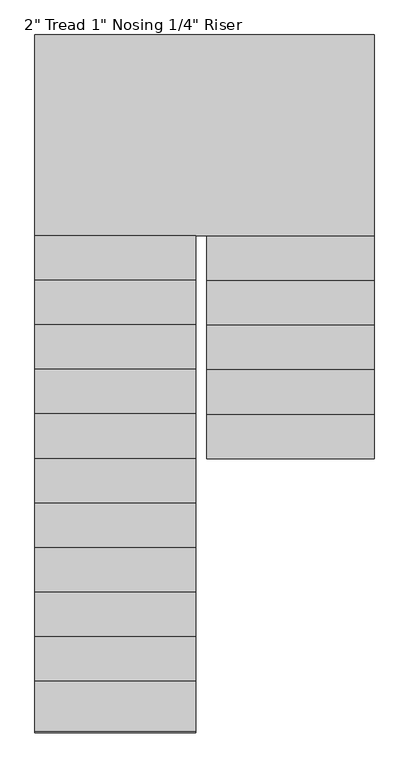
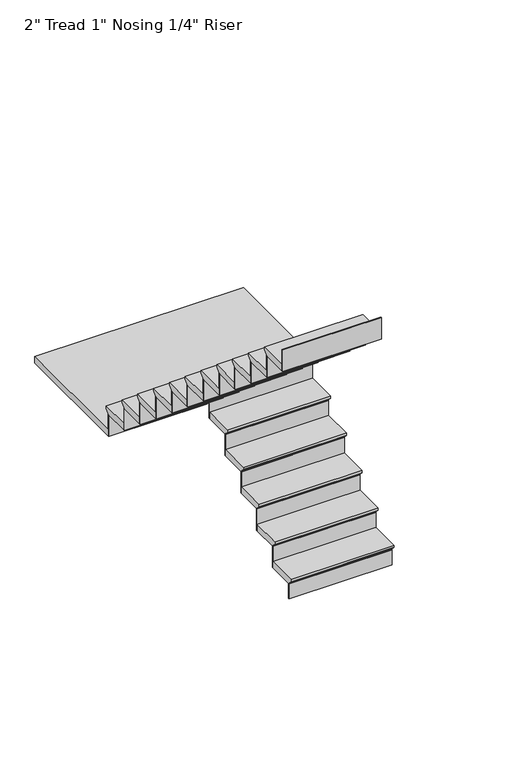
"""IFC4 building model written with IfcOpenShell, lengths in millimetres: stair flight geometry."""

from ifc_helpers import new_model, si_unit, origin, place, context, project, spatial, faceted_brep, source, transform, mapped, element, save


def stair_flight_2b9b7e9b(model_context):
    return source(origin(), model_context, "Body", "Brep", [
        faceted_brep([(-3749.597125, 2714.6319226, 150.2833333), (-3749.597125, 2714.6319226, 169.3333333), (-4512.2136682, 2714.6319226, 169.3333333), (-4512.2136682, 2714.6319226, 150.2833333), (-3749.597125, 2740.0319226, 124.8833333), (-4512.2136682, 2740.0319226, 124.8833333), (-3749.597125, 2943.2319226, 169.3333333), (-4512.2136682, 2943.2319226, 169.3333333), (-4512.2136682, 2740.0319226, 118.5333333), (-4512.2136682, 2943.2319226, 118.5333333), (-3749.597125, 2943.2319226, 118.5333333), (-3749.597125, 2740.0319226, 118.5333333)], [[[0, 1, 2, 3]], [[4, 0, 3, 5]], [[2, 1, 6, 7]], [[8, 9, 10, 11]], [[2, 7, 9, 8, 5, 3]], [[8, 11, 4, 5]], [[6, 1, 0, 4, 11, 10]], [[7, 6, 10, 9]]]),
        faceted_brep([(-3749.597125, 2740.0319226, 118.5333333), (-3749.597125, 2740.0319226, 0.0), (-3749.597125, 2746.3819226, 0.0), (-3749.597125, 2746.3819226, 118.5333333), (-4512.2136682, 2740.0319226, 118.5333333), (-4512.2136682, 2746.3819226, 118.5333333), (-4512.2136682, 2746.3819226, 0.0), (-4512.2136682, 2740.0319226, 0.0)], [[[0, 1, 2, 3]], [[4, 5, 6, 7]], [[1, 0, 4, 7]], [[2, 1, 7, 6]], [[3, 2, 6, 5]], [[0, 3, 5, 4]]]),
        faceted_brep([(-3749.597125, 2943.2319226, 287.8666667), (-3749.597125, 2943.2319226, 118.5333333), (-3749.597125, 2949.5819226, 118.5333333), (-3749.597125, 2949.5819226, 287.8666667), (-4512.2136682, 2943.2319226, 287.8666667), (-4512.2136682, 2949.5819226, 287.8666667), (-4512.2136682, 2949.5819226, 118.5333333), (-4512.2136682, 2943.2319226, 118.5333333)], [[[0, 1, 2, 3]], [[4, 5, 6, 7]], [[1, 0, 4, 7]], [[2, 1, 7, 6]], [[3, 2, 6, 5]], [[0, 3, 5, 4]]]),
        faceted_brep([(-4512.2136682, 2917.8319226, 338.6666667), (-3749.597125, 2917.8319226, 338.6666667), (-3749.597125, 3146.4319226, 338.6666667), (-4512.2136682, 3146.4319226, 338.6666667), (-4512.2136682, 2943.2319226, 287.8666667), (-4512.2136682, 3146.4319226, 287.8666667), (-3749.597125, 3146.4319226, 287.8666667), (-3749.597125, 2943.2319226, 287.8666667), (-4512.2136682, 2943.2319226, 294.2166667), (-4512.2136682, 2917.8319226, 319.6166667), (-3749.597125, 2943.2319226, 294.2166667), (-3749.597125, 2917.8319226, 319.6166667)], [[[0, 1, 2, 3]], [[4, 5, 6, 7]], [[0, 3, 5, 4, 8, 9]], [[4, 7, 10, 8]], [[2, 1, 11, 10, 7, 6]], [[3, 2, 6, 5]], [[11, 1, 0, 9]], [[10, 11, 9, 8]]]),
        faceted_brep([(-3749.597125, 3146.4319226, 457.2), (-3749.597125, 3146.4319226, 287.8666667), (-3749.597125, 3152.7819226, 287.8666667), (-3749.597125, 3152.7819226, 457.2), (-4512.2136682, 3146.4319226, 457.2), (-4512.2136682, 3152.7819226, 457.2), (-4512.2136682, 3152.7819226, 287.8666667), (-4512.2136682, 3146.4319226, 287.8666667)], [[[0, 1, 2, 3]], [[4, 5, 6, 7]], [[1, 0, 4, 7]], [[2, 1, 7, 6]], [[3, 2, 6, 5]], [[0, 3, 5, 4]]]),
        faceted_brep([(-4512.2136682, 3121.0319226, 508.0), (-3749.597125, 3121.0319226, 508.0), (-3749.597125, 3349.6319226, 508.0), (-4512.2136682, 3349.6319226, 508.0), (-4512.2136682, 3146.4319226, 457.2), (-4512.2136682, 3349.6319226, 457.2), (-3749.597125, 3349.6319226, 457.2), (-3749.597125, 3146.4319226, 457.2), (-4512.2136682, 3146.4319226, 463.55), (-4512.2136682, 3121.0319226, 488.95), (-3749.597125, 3146.4319226, 463.55), (-3749.597125, 3121.0319226, 488.95)], [[[0, 1, 2, 3]], [[4, 5, 6, 7]], [[0, 3, 5, 4, 8, 9]], [[4, 7, 10, 8]], [[2, 1, 11, 10, 7, 6]], [[3, 2, 6, 5]], [[11, 1, 0, 9]], [[10, 11, 9, 8]]]),
        faceted_brep([(-3749.597125, 3349.6319226, 626.5333333), (-3749.597125, 3349.6319226, 457.2), (-3749.597125, 3355.9819226, 457.2), (-3749.597125, 3355.9819226, 626.5333333), (-4512.2136682, 3349.6319226, 626.5333333), (-4512.2136682, 3355.9819226, 626.5333333), (-4512.2136682, 3355.9819226, 457.2), (-4512.2136682, 3349.6319226, 457.2)], [[[0, 1, 2, 3]], [[4, 5, 6, 7]], [[1, 0, 4, 7]], [[2, 1, 7, 6]], [[3, 2, 6, 5]], [[0, 3, 5, 4]]]),
        faceted_brep([(-4512.2136682, 3324.2319226, 677.3333333), (-3749.597125, 3324.2319226, 677.3333333), (-3749.597125, 3552.8319226, 677.3333333), (-4512.2136682, 3552.8319226, 677.3333333), (-4512.2136682, 3349.6319226, 626.5333333), (-4512.2136682, 3552.8319226, 626.5333333), (-3749.597125, 3552.8319226, 626.5333333), (-3749.597125, 3349.6319226, 626.5333333), (-4512.2136682, 3349.6319226, 632.8833333), (-4512.2136682, 3324.2319226, 658.2833333), (-3749.597125, 3349.6319226, 632.8833333), (-3749.597125, 3324.2319226, 658.2833333)], [[[0, 1, 2, 3]], [[4, 5, 6, 7]], [[0, 3, 5, 4, 8, 9]], [[4, 7, 10, 8]], [[2, 1, 11, 10, 7, 6]], [[3, 2, 6, 5]], [[11, 1, 0, 9]], [[10, 11, 9, 8]]]),
        faceted_brep([(-3749.597125, 3552.8319226, 795.8666667), (-3749.597125, 3552.8319226, 626.5333333), (-3749.597125, 3559.1819226, 626.5333333), (-3749.597125, 3559.1819226, 795.8666667), (-4512.2136682, 3552.8319226, 795.8666667), (-4512.2136682, 3559.1819226, 795.8666667), (-4512.2136682, 3559.1819226, 626.5333333), (-4512.2136682, 3552.8319226, 626.5333333)], [[[0, 1, 2, 3]], [[4, 5, 6, 7]], [[1, 0, 4, 7]], [[2, 1, 7, 6]], [[3, 2, 6, 5]], [[0, 3, 5, 4]]]),
        faceted_brep([(-4512.2136682, 3527.4319226, 846.6666667), (-3749.597125, 3527.4319226, 846.6666667), (-3749.597125, 3756.0319226, 846.6666667), (-4512.2136682, 3756.0319226, 846.6666667), (-4512.2136682, 3552.8319226, 795.8666667), (-4512.2136682, 3756.0319226, 795.8666667), (-3749.597125, 3756.0319226, 795.8666667), (-3749.597125, 3552.8319226, 795.8666667), (-4512.2136682, 3552.8319226, 802.2166667), (-4512.2136682, 3527.4319226, 827.6166667), (-3749.597125, 3552.8319226, 802.2166667), (-3749.597125, 3527.4319226, 827.6166667)], [[[0, 1, 2, 3]], [[4, 5, 6, 7]], [[0, 3, 5, 4, 8, 9]], [[4, 7, 10, 8]], [[2, 1, 11, 10, 7, 6]], [[3, 2, 6, 5]], [[11, 1, 0, 9]], [[10, 11, 9, 8]]]),
        faceted_brep([(-3749.597125, 3756.0319226, 965.2), (-3749.597125, 3756.0319226, 795.8666667), (-3749.597125, 3762.3819226, 795.8666667), (-3749.597125, 3762.3819226, 965.2), (-4512.2136682, 3756.0319226, 965.2), (-4512.2136682, 3762.3819226, 965.2), (-4512.2136682, 3762.3819226, 795.8666667), (-4512.2136682, 3756.0319226, 795.8666667)], [[[0, 1, 2, 3]], [[4, 5, 6, 7]], [[1, 0, 4, 7]], [[2, 1, 7, 6]], [[3, 2, 6, 5]], [[0, 3, 5, 4]]]),
        faceted_brep([(-4563.0136682, 3705.2319226, 1016.0), (-4563.0136682, 3730.6319226, 1016.0), (-3749.597125, 3730.6319226, 1016.0), (-3749.597125, 4645.0319226, 1016.0), (-5295.0246464, 4645.0319226, 1016.0), (-5295.0246464, 3705.2319226, 1016.0), (-4563.0136682, 3730.6319226, 965.2), (-4563.0136682, 3705.2319226, 965.2), (-5295.0246464, 3705.2319226, 965.2), (-5295.0246464, 4645.0319226, 965.2), (-3749.597125, 4645.0319226, 965.2), (-3749.597125, 3756.0319226, 965.2), (-4512.2136682, 3756.0319226, 965.2), (-4512.2136682, 3730.6319226, 965.2), (-4512.2136682, 3730.6319226, 996.95), (-3749.597125, 3730.6319226, 996.95), (-4512.2136682, 3756.0319226, 971.55), (-3749.597125, 3756.0319226, 971.55)], [[[0, 1, 2, 3, 4, 5]], [[6, 7, 8, 9, 10, 11, 12, 13]], [[1, 0, 7, 6]], [[2, 1, 6, 13, 14, 15]], [[13, 12, 16, 14]], [[12, 11, 17, 16]], [[3, 2, 15, 17, 11, 10]], [[4, 3, 10, 9]], [[5, 4, 9, 8]], [[0, 5, 8, 7]], [[17, 15, 14, 16]]]),
        faceted_brep([(-5295.0246464, 3705.2319226, 1134.5333333), (-5295.0246464, 3705.2319226, 965.2), (-5295.0246464, 3698.8819226, 965.2), (-5295.0246464, 3698.8819226, 1134.5333333), (-4563.0136682, 3705.2319226, 1134.5333333), (-4563.0136682, 3698.8819226, 1134.5333333), (-4563.0136682, 3698.8819226, 965.2), (-4563.0136682, 3705.2319226, 965.2)], [[[0, 1, 2, 3]], [[4, 5, 6, 7]], [[1, 0, 4, 7]], [[2, 1, 7, 6]], [[3, 2, 6, 5]], [[0, 3, 5, 4]]]),
        faceted_brep([(-4563.0136682, 3730.6319226, 1185.3333333), (-5295.0246464, 3730.6319226, 1185.3333333), (-5295.0246464, 3502.0319226, 1185.3333333), (-4563.0136682, 3502.0319226, 1185.3333333), (-4563.0136682, 3705.2319226, 1134.5333333), (-4563.0136682, 3502.0319226, 1134.5333333), (-5295.0246464, 3502.0319226, 1134.5333333), (-5295.0246464, 3705.2319226, 1134.5333333), (-4563.0136682, 3705.2319226, 1140.8833333), (-4563.0136682, 3730.6319226, 1166.2833333), (-5295.0246464, 3705.2319226, 1140.8833333), (-5295.0246464, 3730.6319226, 1166.2833333)], [[[0, 1, 2, 3]], [[4, 5, 6, 7]], [[0, 3, 5, 4, 8, 9]], [[4, 7, 10, 8]], [[2, 1, 11, 10, 7, 6]], [[3, 2, 6, 5]], [[11, 1, 0, 9]], [[10, 11, 9, 8]]]),
        faceted_brep([(-5295.0246464, 3502.0319226, 1303.8666667), (-5295.0246464, 3502.0319226, 1134.5333333), (-5295.0246464, 3495.6819226, 1134.5333333), (-5295.0246464, 3495.6819226, 1303.8666667), (-4563.0136682, 3502.0319226, 1303.8666667), (-4563.0136682, 3495.6819226, 1303.8666667), (-4563.0136682, 3495.6819226, 1134.5333333), (-4563.0136682, 3502.0319226, 1134.5333333)], [[[0, 1, 2, 3]], [[4, 5, 6, 7]], [[1, 0, 4, 7]], [[2, 1, 7, 6]], [[3, 2, 6, 5]], [[0, 3, 5, 4]]]),
        faceted_brep([(-4563.0136682, 3527.4319226, 1354.6666667), (-5295.0246464, 3527.4319226, 1354.6666667), (-5295.0246464, 3298.8319226, 1354.6666667), (-4563.0136682, 3298.8319226, 1354.6666667), (-4563.0136682, 3502.0319226, 1303.8666667), (-4563.0136682, 3298.8319226, 1303.8666667), (-5295.0246464, 3298.8319226, 1303.8666667), (-5295.0246464, 3502.0319226, 1303.8666667), (-4563.0136682, 3502.0319226, 1310.2166667), (-4563.0136682, 3527.4319226, 1335.6166667), (-5295.0246464, 3502.0319226, 1310.2166667), (-5295.0246464, 3527.4319226, 1335.6166667)], [[[0, 1, 2, 3]], [[4, 5, 6, 7]], [[0, 3, 5, 4, 8, 9]], [[4, 7, 10, 8]], [[2, 1, 11, 10, 7, 6]], [[3, 2, 6, 5]], [[11, 1, 0, 9]], [[10, 11, 9, 8]]]),
        faceted_brep([(-5295.0246464, 3298.8319226, 1473.2), (-5295.0246464, 3298.8319226, 1303.8666667), (-5295.0246464, 3292.4819226, 1303.8666667), (-5295.0246464, 3292.4819226, 1473.2), (-4563.0136682, 3298.8319226, 1473.2), (-4563.0136682, 3292.4819226, 1473.2), (-4563.0136682, 3292.4819226, 1303.8666667), (-4563.0136682, 3298.8319226, 1303.8666667)], [[[0, 1, 2, 3]], [[4, 5, 6, 7]], [[1, 0, 4, 7]], [[2, 1, 7, 6]], [[3, 2, 6, 5]], [[0, 3, 5, 4]]]),
        faceted_brep([(-4563.0136682, 3324.2319226, 1524.0), (-5295.0246464, 3324.2319226, 1524.0), (-5295.0246464, 3095.6319226, 1524.0), (-4563.0136682, 3095.6319226, 1524.0), (-4563.0136682, 3298.8319226, 1473.2), (-4563.0136682, 3095.6319226, 1473.2), (-5295.0246464, 3095.6319226, 1473.2), (-5295.0246464, 3298.8319226, 1473.2), (-4563.0136682, 3298.8319226, 1479.55), (-4563.0136682, 3324.2319226, 1504.95), (-5295.0246464, 3298.8319226, 1479.55), (-5295.0246464, 3324.2319226, 1504.95)], [[[0, 1, 2, 3]], [[4, 5, 6, 7]], [[0, 3, 5, 4, 8, 9]], [[4, 7, 10, 8]], [[2, 1, 11, 10, 7, 6]], [[3, 2, 6, 5]], [[11, 1, 0, 9]], [[10, 11, 9, 8]]]),
        faceted_brep([(-5295.0246464, 3095.6319226, 1642.5333333), (-5295.0246464, 3095.6319226, 1473.2), (-5295.0246464, 3089.2819226, 1473.2), (-5295.0246464, 3089.2819226, 1642.5333333), (-4563.0136682, 3095.6319226, 1642.5333333), (-4563.0136682, 3089.2819226, 1642.5333333), (-4563.0136682, 3089.2819226, 1473.2), (-4563.0136682, 3095.6319226, 1473.2)], [[[0, 1, 2, 3]], [[4, 5, 6, 7]], [[1, 0, 4, 7]], [[2, 1, 7, 6]], [[3, 2, 6, 5]], [[0, 3, 5, 4]]]),
        faceted_brep([(-4563.0136682, 3121.0319226, 1693.3333333), (-5295.0246464, 3121.0319226, 1693.3333333), (-5295.0246464, 2892.4319226, 1693.3333333), (-4563.0136682, 2892.4319226, 1693.3333333), (-4563.0136682, 3095.6319226, 1642.5333333), (-4563.0136682, 2892.4319226, 1642.5333333), (-5295.0246464, 2892.4319226, 1642.5333333), (-5295.0246464, 3095.6319226, 1642.5333333), (-4563.0136682, 3095.6319226, 1648.8833333), (-4563.0136682, 3121.0319226, 1674.2833333), (-5295.0246464, 3095.6319226, 1648.8833333), (-5295.0246464, 3121.0319226, 1674.2833333)], [[[0, 1, 2, 3]], [[4, 5, 6, 7]], [[0, 3, 5, 4, 8, 9]], [[4, 7, 10, 8]], [[2, 1, 11, 10, 7, 6]], [[3, 2, 6, 5]], [[11, 1, 0, 9]], [[10, 11, 9, 8]]]),
        faceted_brep([(-5295.0246464, 2892.4319226, 1811.8666667), (-5295.0246464, 2892.4319226, 1642.5333333), (-5295.0246464, 2886.0819226, 1642.5333333), (-5295.0246464, 2886.0819226, 1811.8666667), (-4563.0136682, 2892.4319226, 1811.8666667), (-4563.0136682, 2886.0819226, 1811.8666667), (-4563.0136682, 2886.0819226, 1642.5333333), (-4563.0136682, 2892.4319226, 1642.5333333)], [[[0, 1, 2, 3]], [[4, 5, 6, 7]], [[1, 0, 4, 7]], [[2, 1, 7, 6]], [[3, 2, 6, 5]], [[0, 3, 5, 4]]]),
        faceted_brep([(-4563.0136682, 2917.8319226, 1862.6666667), (-5295.0246464, 2917.8319226, 1862.6666667), (-5295.0246464, 2689.2319226, 1862.6666667), (-4563.0136682, 2689.2319226, 1862.6666667), (-4563.0136682, 2892.4319226, 1811.8666667), (-4563.0136682, 2689.2319226, 1811.8666667), (-5295.0246464, 2689.2319226, 1811.8666667), (-5295.0246464, 2892.4319226, 1811.8666667), (-4563.0136682, 2892.4319226, 1818.2166667), (-4563.0136682, 2917.8319226, 1843.6166667), (-5295.0246464, 2892.4319226, 1818.2166667), (-5295.0246464, 2917.8319226, 1843.6166667)], [[[0, 1, 2, 3]], [[4, 5, 6, 7]], [[0, 3, 5, 4, 8, 9]], [[4, 7, 10, 8]], [[2, 1, 11, 10, 7, 6]], [[3, 2, 6, 5]], [[11, 1, 0, 9]], [[10, 11, 9, 8]]]),
        faceted_brep([(-5295.0246464, 2689.2319226, 1981.2), (-5295.0246464, 2689.2319226, 1811.8666667), (-5295.0246464, 2682.8819226, 1811.8666667), (-5295.0246464, 2682.8819226, 1981.2), (-4563.0136682, 2689.2319226, 1981.2), (-4563.0136682, 2682.8819226, 1981.2), (-4563.0136682, 2682.8819226, 1811.8666667), (-4563.0136682, 2689.2319226, 1811.8666667)], [[[0, 1, 2, 3]], [[4, 5, 6, 7]], [[1, 0, 4, 7]], [[2, 1, 7, 6]], [[3, 2, 6, 5]], [[0, 3, 5, 4]]]),
        faceted_brep([(-4563.0136682, 2714.6319226, 2032.0), (-5295.0246464, 2714.6319226, 2032.0), (-5295.0246464, 2486.0319226, 2032.0), (-4563.0136682, 2486.0319226, 2032.0), (-4563.0136682, 2689.2319226, 1981.2), (-4563.0136682, 2486.0319226, 1981.2), (-5295.0246464, 2486.0319226, 1981.2), (-5295.0246464, 2689.2319226, 1981.2), (-4563.0136682, 2689.2319226, 1987.55), (-4563.0136682, 2714.6319226, 2012.95), (-5295.0246464, 2689.2319226, 1987.55), (-5295.0246464, 2714.6319226, 2012.95)], [[[0, 1, 2, 3]], [[4, 5, 6, 7]], [[0, 3, 5, 4, 8, 9]], [[4, 7, 10, 8]], [[2, 1, 11, 10, 7, 6]], [[3, 2, 6, 5]], [[11, 1, 0, 9]], [[10, 11, 9, 8]]]),
        faceted_brep([(-5295.0246464, 2486.0319226, 2150.5333333), (-5295.0246464, 2486.0319226, 1981.2), (-5295.0246464, 2479.6819226, 1981.2), (-5295.0246464, 2479.6819226, 2150.5333333), (-4563.0136682, 2486.0319226, 2150.5333333), (-4563.0136682, 2479.6819226, 2150.5333333), (-4563.0136682, 2479.6819226, 1981.2), (-4563.0136682, 2486.0319226, 1981.2)], [[[0, 1, 2, 3]], [[4, 5, 6, 7]], [[1, 0, 4, 7]], [[2, 1, 7, 6]], [[3, 2, 6, 5]], [[0, 3, 5, 4]]]),
        faceted_brep([(-4563.0136682, 2511.4319226, 2201.3333333), (-5295.0246464, 2511.4319226, 2201.3333333), (-5295.0246464, 2282.8319226, 2201.3333333), (-4563.0136682, 2282.8319226, 2201.3333333), (-4563.0136682, 2486.0319226, 2150.5333333), (-4563.0136682, 2282.8319226, 2150.5333333), (-5295.0246464, 2282.8319226, 2150.5333333), (-5295.0246464, 2486.0319226, 2150.5333333), (-4563.0136682, 2486.0319226, 2156.8833333), (-4563.0136682, 2511.4319226, 2182.2833333), (-5295.0246464, 2486.0319226, 2156.8833333), (-5295.0246464, 2511.4319226, 2182.2833333)], [[[0, 1, 2, 3]], [[4, 5, 6, 7]], [[0, 3, 5, 4, 8, 9]], [[4, 7, 10, 8]], [[2, 1, 11, 10, 7, 6]], [[3, 2, 6, 5]], [[11, 1, 0, 9]], [[10, 11, 9, 8]]]),
        faceted_brep([(-5295.0246464, 2282.8319226, 2319.8666667), (-5295.0246464, 2282.8319226, 2150.5333333), (-5295.0246464, 2276.4819226, 2150.5333333), (-5295.0246464, 2276.4819226, 2319.8666667), (-4563.0136682, 2282.8319226, 2319.8666667), (-4563.0136682, 2276.4819226, 2319.8666667), (-4563.0136682, 2276.4819226, 2150.5333333), (-4563.0136682, 2282.8319226, 2150.5333333)], [[[0, 1, 2, 3]], [[4, 5, 6, 7]], [[1, 0, 4, 7]], [[2, 1, 7, 6]], [[3, 2, 6, 5]], [[0, 3, 5, 4]]]),
        faceted_brep([(-4563.0136682, 2308.2319226, 2370.6666667), (-5295.0246464, 2308.2319226, 2370.6666667), (-5295.0246464, 2079.6319226, 2370.6666667), (-4563.0136682, 2079.6319226, 2370.6666667), (-4563.0136682, 2282.8319226, 2319.8666667), (-4563.0136682, 2079.6319226, 2319.8666667), (-5295.0246464, 2079.6319226, 2319.8666667), (-5295.0246464, 2282.8319226, 2319.8666667), (-4563.0136682, 2282.8319226, 2326.2166667), (-4563.0136682, 2308.2319226, 2351.6166667), (-5295.0246464, 2282.8319226, 2326.2166667), (-5295.0246464, 2308.2319226, 2351.6166667)], [[[0, 1, 2, 3]], [[4, 5, 6, 7]], [[0, 3, 5, 4, 8, 9]], [[4, 7, 10, 8]], [[2, 1, 11, 10, 7, 6]], [[3, 2, 6, 5]], [[11, 1, 0, 9]], [[10, 11, 9, 8]]]),
        faceted_brep([(-5295.0246464, 2079.6319226, 2489.2), (-5295.0246464, 2079.6319226, 2319.8666667), (-5295.0246464, 2073.2819226, 2319.8666667), (-5295.0246464, 2073.2819226, 2489.2), (-4563.0136682, 2079.6319226, 2489.2), (-4563.0136682, 2073.2819226, 2489.2), (-4563.0136682, 2073.2819226, 2319.8666667), (-4563.0136682, 2079.6319226, 2319.8666667)], [[[0, 1, 2, 3]], [[4, 5, 6, 7]], [[1, 0, 4, 7]], [[2, 1, 7, 6]], [[3, 2, 6, 5]], [[0, 3, 5, 4]]]),
        faceted_brep([(-4563.0136682, 2105.0319226, 2540.0), (-5295.0246464, 2105.0319226, 2540.0), (-5295.0246464, 1876.4319226, 2540.0), (-4563.0136682, 1876.4319226, 2540.0), (-4563.0136682, 2079.6319226, 2489.2), (-4563.0136682, 1876.4319226, 2489.2), (-5295.0246464, 1876.4319226, 2489.2), (-5295.0246464, 2079.6319226, 2489.2), (-4563.0136682, 2079.6319226, 2495.55), (-4563.0136682, 2105.0319226, 2520.95), (-5295.0246464, 2079.6319226, 2495.55), (-5295.0246464, 2105.0319226, 2520.95)], [[[0, 1, 2, 3]], [[4, 5, 6, 7]], [[0, 3, 5, 4, 8, 9]], [[4, 7, 10, 8]], [[2, 1, 11, 10, 7, 6]], [[3, 2, 6, 5]], [[11, 1, 0, 9]], [[10, 11, 9, 8]]]),
        faceted_brep([(-5295.0246464, 1876.4319226, 2658.5333333), (-5295.0246464, 1876.4319226, 2489.2), (-5295.0246464, 1870.0819226, 2489.2), (-5295.0246464, 1870.0819226, 2658.5333333), (-4563.0136682, 1876.4319226, 2658.5333333), (-4563.0136682, 1870.0819226, 2658.5333333), (-4563.0136682, 1870.0819226, 2489.2), (-4563.0136682, 1876.4319226, 2489.2)], [[[0, 1, 2, 3]], [[4, 5, 6, 7]], [[1, 0, 4, 7]], [[2, 1, 7, 6]], [[3, 2, 6, 5]], [[0, 3, 5, 4]]]),
        faceted_brep([(-4563.0136682, 1901.8319226, 2709.3333333), (-5295.0246464, 1901.8319226, 2709.3333333), (-5295.0246464, 1673.2319226, 2709.3333333), (-4563.0136682, 1673.2319226, 2709.3333333), (-4563.0136682, 1876.4319226, 2658.5333333), (-4563.0136682, 1673.2319226, 2658.5333333), (-5295.0246464, 1673.2319226, 2658.5333333), (-5295.0246464, 1876.4319226, 2658.5333333), (-4563.0136682, 1876.4319226, 2664.8833333), (-4563.0136682, 1901.8319226, 2690.2833333), (-5295.0246464, 1876.4319226, 2664.8833333), (-5295.0246464, 1901.8319226, 2690.2833333)], [[[0, 1, 2, 3]], [[4, 5, 6, 7]], [[0, 3, 5, 4, 8, 9]], [[4, 7, 10, 8]], [[2, 1, 11, 10, 7, 6]], [[3, 2, 6, 5]], [[11, 1, 0, 9]], [[10, 11, 9, 8]]]),
        faceted_brep([(-5295.0246464, 1673.2319226, 2827.8666667), (-5295.0246464, 1673.2319226, 2658.5333333), (-5295.0246464, 1666.8819226, 2658.5333333), (-5295.0246464, 1666.8819226, 2827.8666667), (-4563.0136682, 1673.2319226, 2827.8666667), (-4563.0136682, 1666.8819226, 2827.8666667), (-4563.0136682, 1666.8819226, 2658.5333333), (-4563.0136682, 1673.2319226, 2658.5333333)], [[[0, 1, 2, 3]], [[4, 5, 6, 7]], [[1, 0, 4, 7]], [[2, 1, 7, 6]], [[3, 2, 6, 5]], [[0, 3, 5, 4]]]),
        faceted_brep([(-4563.0136682, 1698.6319226, 2878.6666667), (-5295.0246464, 1698.6319226, 2878.6666667), (-5295.0246464, 1470.0319226, 2878.6666667), (-4563.0136682, 1470.0319226, 2878.6666667), (-4563.0136682, 1673.2319226, 2827.8666667), (-4563.0136682, 1470.0319226, 2827.8666667), (-5295.0246464, 1470.0319226, 2827.8666667), (-5295.0246464, 1673.2319226, 2827.8666667), (-4563.0136682, 1673.2319226, 2834.2166667), (-4563.0136682, 1698.6319226, 2859.6166667), (-5295.0246464, 1673.2319226, 2834.2166667), (-5295.0246464, 1698.6319226, 2859.6166667)], [[[0, 1, 2, 3]], [[4, 5, 6, 7]], [[0, 3, 5, 4, 8, 9]], [[4, 7, 10, 8]], [[2, 1, 11, 10, 7, 6]], [[3, 2, 6, 5]], [[11, 1, 0, 9]], [[10, 11, 9, 8]]]),
        faceted_brep([(-5295.0246464, 1470.0319226, 2997.2), (-5295.0246464, 1470.0319226, 2827.8666667), (-5295.0246464, 1463.6819226, 2827.8666667), (-5295.0246464, 1463.6819226, 2997.2), (-4563.0136682, 1470.0319226, 2997.2), (-4563.0136682, 1463.6819226, 2997.2), (-4563.0136682, 1463.6819226, 2827.8666667), (-4563.0136682, 1470.0319226, 2827.8666667)], [[[0, 1, 2, 3]], [[4, 5, 6, 7]], [[1, 0, 4, 7]], [[2, 1, 7, 6]], [[3, 2, 6, 5]], [[0, 3, 5, 4]]]),
    ])


if __name__ == "__main__":
    model = new_model("IFC4")
    model_context = context("Model", 3, world=origin())
    ifc_project = project(units=[si_unit("LENGTHUNIT", "METRE", prefix="MILLI")], contexts=[model_context])
    site = spatial("IfcSite", under=ifc_project)
    building = spatial("IfcBuilding", under=site)
    placement = place(None, origin())
    stair_flight_shape = stair_flight_2b9b7e9b(model_context)
    element("IfcStairFlight", 1, ObjectType="2\" Tread 1\" Nosing 1/4\" Riser", at=placement, inside=building, context=model_context, shape_type="MappedRepresentation", body=[
        mapped(stair_flight_shape, transform((0.0, 0.0, 0.0), x_axis=(1.0, 0.0, 0.0), y_axis=(0.0, 1.0, 0.0), z_axis=(0.0, 0.0, 1.0))),
    ])
    save(model, "model.ifc")
